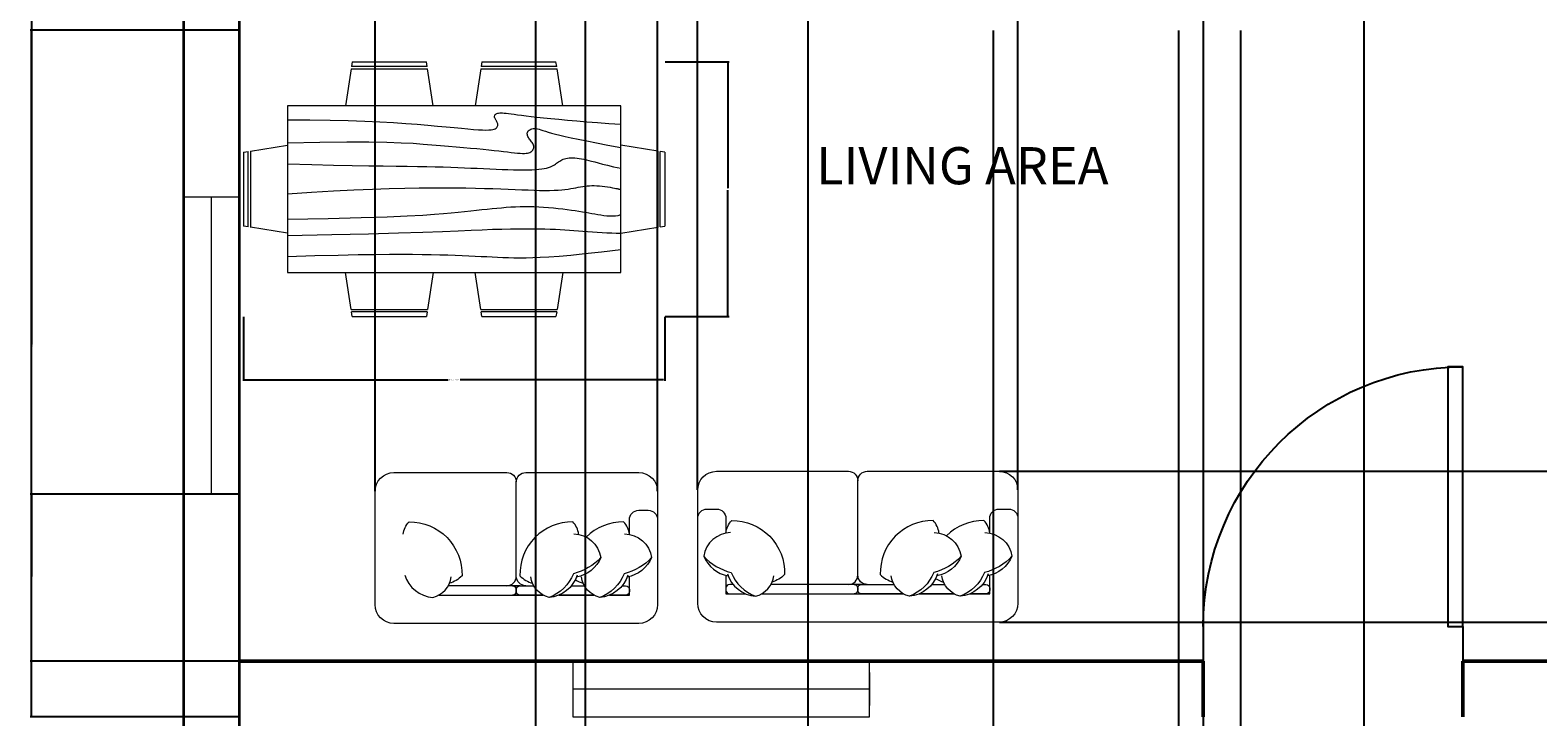
# Model space of a CAD drawing. Units: inches. Extents: x 8049 to 8459, y 820 to 1350.
# Tile 22 of 25: x 8050 to 8294, y 1046 to 1157. Entities that reach past the tile are written whole.
import ezdxf

# ---------------------------------------------------------------- set-up
doc = ezdxf.new("R2010")
doc.units = ezdxf.units.IN
doc.header["$MEASUREMENT"] = 0
for name, color, linetype, lineweight in [('A-ANNO-DIMS', 2, 'Continuous', 18), ('A-AREA-IDEN', 7, 'Continuous', 25), ('A-DOOR', 3, 'Continuous', 25), ('A-FURN', 8, 'Continuous', 18), ('A-GLAZ', 4, 'Continuous', 18), ('A-WALL', 7, 'Continuous', 50), ('C-SITE-WALL', 7, 'Continuous', 35)]:
    doc.layers.add(name, color=color, linetype=linetype, lineweight=lineweight)
doc.styles.get("Standard").update_dxf_attribs({"font": 'arial.ttf'})
doc.dimstyles.get("Standard").update_dxf_attribs({"dimtxt": 0.18, "dimasz": 0.18, "dimexe": 0.18, "dimexo": 0.0625, "dimgap": 0.09, "dimtad": 0, "dimtih": 1, "dimtoh": 1, "dimdec": 4, "dimzin": 0, "dimdsep": 46, "dimtxsty": 'Standard', "dimcen": 0.09, "dimadec": 0, "dimazin": 0, "dimtfac": 1, "dimtdec": 4, "dimtofl": 0, "dimtmove": 0, "dimatfit": 3, "dimfxl": 1, "dimtolj": 1, "dimtzin": 0, "dimarcsym": 0})

# ---------------------------------------------------------------- blocks, each defined once
blk = doc.blocks.new('*U2')
for p, q in [((0, 0), (0, -100)), ((750, 0), (750, -100))]:
    blk.add_line(p, q)
blk.add_lwpolyline([(0, 0), (0, 750), (43.75, 750), (43.75, 0)], close=True)
blk.add_arc((0, 0), 750, 0, 90)
blk = doc.blocks.new('*U4')
for p, q in [((0, 100), (0, 0)), ((900, 100), (900, 0)), ((0, 50), (900, 50))]:
    blk.add_line(p, q)
blk = doc.blocks.new('Dining Set - 36 x 72 in.')
for p, q in [((-22, 27.5), (-22.1562, 26.50042)), ((-5.8416, 26.5), (-22.1534, 26.5)), ((-22, 27.5), (-6, 27.5)), ((-5.8437, 26.49966), (-6, 27.5)), ((6, 27.5), (5.8438, 26.50042)), ((22.1584, 26.5), (5.8466, 26.5)), ((6, 27.5), (22, 27.5)), ((22.1563, 26.49966), (22, 27.5)), ((-22.2343, 26.00059), (-23.4847, 17.99762)), ((-22.2304, 26), (-5.7608, 26)), ((-4.5152, 17.99762), (-5.7655, 25.99926)), ((5.7657, 26.00059), (4.5153, 17.99762)), ((5.7696, 26), (22.2392, 26)), ((23.4848, 17.99762), (22.2345, 25.99926)), ((36, 18), (-36, 18)), ((-36, 18), (-36, -18)), ((36, -18), (36, 18)), ((-45.5, 8), (-44.5004, 8.15617)), ((-45.5, 8), (-45.5, -8)), ((-44.5, -8.15843), (-44.5, 8.15338)), ((-44.0006, 8.23428), (-35.9976, 9.48474)), ((-44, 8.23041), (-44, -8.23915)), ((44.0006, 8.23428), (35.9976, 9.48474)), ((44, 8.23041), (44, -8.23915)), ((44.5, -8.15843), (44.5, 8.15338)), ((45.5, 8), (44.5005, 8.15617)), ((45.5, 8), (45.5, -8)), ((-44.4997, -8.15631), (-45.5, -8)), ((-35.9976, -9.48476), (-43.9993, -8.2345)), ((35.9976, -9.48476), (43.9993, -8.2345)), ((44.4997, -8.15631), (45.5, -8)), ((-36, -18), (36, -18)), ((-22.2343, -26.0006), (-23.4847, -17.99762)), ((-4.5152, -17.99762), (-5.7655, -25.99928)), ((5.7657, -26.0006), (4.5153, -17.99762)), ((23.4848, -17.99762), (22.2345, -25.99928)), ((-22.2304, -26), (-5.7608, -26)), ((5.7696, -26), (22.2392, -26)), ((-22, -27.5), (-22.1562, -26.50044)), ((-5.8416, -26.5), (-22.1534, -26.5)), ((-22, -27.5), (-6, -27.5)), ((-5.8437, -26.49967), (-6, -27.5)), ((6, -27.5), (5.8438, -26.50044)), ((22.1584, -26.5), (5.8466, -26.5)), ((6, -27.5), (22, -27.5)), ((22.1563, -26.49967), (22, -27.5))]:
    blk.add_line(p, q)
for points in [[(-36, 15), (-31.1772, 14.97754), (-26.8079, 14.91406), (-22.8538, 14.81543), (-19.276, 14.6875), (-16.0362, 14.53613), (-13.0957, 14.36718), (-10.4159, 14.18652), (-7.9583, 14), (-5.6904, 13.81315), (-3.6035, 13.63021), (-1.6954, 13.45508), (0.0365, 13.29166), (1.5945, 13.14388), (2.9811, 13.01562), (4.1988, 12.9108), (5.25, 12.83333), (6.1393, 12.78613), (6.8802, 12.76823), (7.4883, 12.77767), (7.9792, 12.8125), (8.3685, 12.87077), (8.6719, 12.95052), (8.9049, 13.0498), (9.0833, 13.16666), (9.2205, 13.29899), (9.3216, 13.44401), (9.3895, 13.59879), (9.4271, 13.76041), (9.4373, 13.92594), (9.4232, 14.09245), (9.3875, 14.257), (9.3333, 14.41666), (9.2638, 14.56917), (9.1836, 14.71484), (9.0975, 14.85465), (9.0104, 14.98958), (8.9272, 15.1206), (8.8529, 15.2487), (8.7922, 15.37483), (8.75, 15.5), (8.7305, 15.62467), (8.7344, 15.74739), (8.7617, 15.86621), (8.8125, 15.97916), (8.8867, 16.08431), (8.9844, 16.17968), (9.1055, 16.26334), (9.25, 16.33333), (9.4189, 16.38802), (9.6172, 16.42708), (9.8506, 16.45052), (10.125, 16.45833), (10.4463, 16.45052), (10.8203, 16.42708), (11.2529, 16.38802), (11.75, 16.33333), (12.3184, 16.26318), (12.9694, 16.17838), (13.7151, 16.07991), (14.5677, 15.96875), (15.5395, 15.84586), (16.6426, 15.71224), (17.8893, 15.56884), (19.2917, 15.41666), (20.859, 15.25667), (22.5879, 15.08984), (24.4721, 14.91715), (26.5052, 14.73958), (28.6809, 14.5581), (30.9929, 14.3737), (33.4347, 14.18733), (36, 14)], [(-36, 10), (-28.9766, 10.14274), (-23.1725, 10.20442), (-18.4241, 10.19775), (-14.5677, 10.13541), (-11.4399, 10.03011), (-8.877, 9.89453), (-6.7154, 9.74137), (-4.7917, 9.58333), (-2.9698, 9.43082), (-1.2246, 9.28515), (0.4415, 9.14534), (2.026, 9.01041), (3.5266, 8.87939), (4.9408, 8.7513), (6.266, 8.62516), (7.5, 8.5), (8.6411, 8.37549), (9.6914, 8.2539), (10.6538, 8.13818), (11.5312, 8.03125), (12.3267, 7.93603), (13.043, 7.85547), (13.6831, 7.79248), (14.25, 7.75), (14.7471, 7.7303), (15.1797, 7.73307), (15.5537, 7.75732), (15.875, 7.80208), (16.1494, 7.86637), (16.3828, 7.94922), (16.5811, 8.04964), (16.75, 8.16666), (16.8944, 8.29915), (17.0143, 8.44531), (17.1089, 8.60319), (17.1771, 8.77083), (17.218, 8.94629), (17.2305, 9.1276), (17.2137, 9.31282), (17.1667, 9.5), (17.0895, 9.6875), (16.987, 9.875), (16.8649, 10.0625), (16.7292, 10.25), (16.5856, 10.4375), (16.4401, 10.625), (16.2985, 10.8125), (16.1667, 11), (16.05, 11.18733), (15.9518, 11.3737), (15.8752, 11.5581), (15.8229, 11.73958), (15.798, 11.91715), (15.8034, 12.08984), (15.842, 12.25667), (15.9167, 12.41666), (16.0295, 12.56836), (16.1784, 12.70833), (16.3605, 12.83268), (16.5729, 12.9375), (16.8127, 13.01888), (17.0768, 13.07291), (17.3625, 13.0957), (17.6667, 13.08333), (17.9894, 13.03312), (18.3418, 12.94726), (18.7382, 12.82918), (19.1927, 12.68229), (19.7195, 12.51001), (20.3327, 12.31575), (21.0465, 12.10294), (21.875, 11.875), (22.8357, 11.63354), (23.959, 11.37304), (25.2786, 11.08618), (26.8282, 10.76562), (28.6414, 10.40405), (30.752, 9.99414), (33.1936, 9.52856), (36, 9)], [(-36, 5.5), (-30.7157, 5.3348), (-26.069, 5.20963), (-21.9946, 5.11767), (-18.4271, 5.05208), (-15.3009, 5.00602), (-12.5508, 4.97265), (-10.1112, 4.94515), (-7.9167, 4.91666), (-5.909, 4.88167), (-4.0586, 4.83984), (-2.3429, 4.79215), (-0.7396, 4.73958), (0.7739, 4.6831), (2.22, 4.6237), (3.6213, 4.56233), (5, 4.5), (6.373, 4.43782), (7.7344, 4.3776), (9.0723, 4.32129), (10.375, 4.27083), (11.6309, 4.22819), (12.8281, 4.19531), (13.9551, 4.17415), (15, 4.16666), (15.954, 4.17448), (16.819, 4.19791), (17.6001, 4.23698), (18.3021, 4.29166), (18.9299, 4.36198), (19.4883, 4.44791), (19.9823, 4.54948), (20.4167, 4.66666), (20.7969, 4.79899), (21.1302, 4.94401), (21.4245, 5.09879), (21.6875, 5.26041), (21.9271, 5.42594), (22.1511, 5.59245), (22.3672, 5.757), (22.5834, 5.91666), (22.8065, 6.06868), (23.0404, 6.21093), (23.2879, 6.34147), (23.5521, 6.45833), (23.8358, 6.55957), (24.142, 6.64323), (24.4735, 6.70735), (24.8334, 6.75), (25.2235, 6.76969), (25.642, 6.76692), (26.0858, 6.74267), (26.5521, 6.69791), (27.0379, 6.63362), (27.5404, 6.55078), (28.0565, 6.45036), (28.5834, 6.33333), (29.1242, 6.19987), (29.7071, 6.04687), (30.3661, 5.87044), (31.1354, 5.66666), (32.0493, 5.43164), (33.142, 5.16146), (34.4475, 4.85221), (36, 4.5)], [(-36, -1), (-30.7915, -0.6591), (-26.0195, -0.38216), (-21.6519, -0.16284), (-17.6563, 0.00521), (-14.0005, 0.12833), (-10.6523, 0.21289), (-7.5796, 0.26522), (-4.75, 0.29166), (-2.134, 0.29793), (0.2878, 0.28711), (2.5317, 0.26163), (4.6146, 0.22396), (6.5529, 0.17651), (8.3633, 0.12174), (10.0623, 0.06209), (11.6667, 0), (13.1899, -0.06201), (14.6341, -0.1211), (15.9982, -0.17432), (17.2813, -0.21875), (18.4823, -0.25147), (19.6003, -0.26953), (20.6343, -0.27002), (21.5834, -0.25), (22.4481, -0.20768), (23.2357, -0.14584), (23.9549, -0.06836), (24.6146, 0.02083), (25.2235, 0.11784), (25.7904, 0.21875), (26.3241, 0.31966), (26.8334, 0.41666), (27.3265, 0.50618), (27.8099, 0.58593), (28.2894, 0.65397), (28.7709, 0.70833), (29.2601, 0.74707), (29.763, 0.76823), (30.2855, 0.76985), (30.8334, 0.75), (31.4088, 0.70784), (31.9994, 0.64713), (32.589, 0.57275), (33.1615, 0.48958), (33.7008, 0.4025), (34.1908, 0.3164), (34.6153, 0.23616), (34.9584, 0.16666), (35.2099, 0.11165), (35.3848, 0.07031), (35.504, 0.04069), (35.5886, 0.02083), (35.6594, 0.00879), (35.7377, 0.0026), (35.8442, 0.00032), (36, 0)], [(-36, -6.5), (-27.1843, -6.31267), (-20.084, -6.1263), (-14.469, -5.9419), (-10.1094, -5.76042), (-6.7752, -5.58285), (-4.2363, -5.41016), (-2.2629, -5.24333), (-0.625, -5.08334), (0.8708, -4.93099), (2.2715, -4.78646), (3.5872, -4.64974), (4.8281, -4.52084), (6.0046, -4.39974), (7.127, -4.28646), (8.2053, -4.18099), (9.25, -4.08334), (10.2705, -3.99382), (11.2734, -3.91407), (12.2647, -3.84603), (13.25, -3.79167), (14.2354, -3.75293), (15.2266, -3.73177), (16.2295, -3.73015), (17.25, -3.75), (18.2912, -3.79248), (19.3451, -3.85547), (20.4009, -3.93604), (21.4479, -4.03125), (22.4754, -4.13819), (23.4727, -4.25391), (24.4289, -4.37549), (25.3334, -4.5), (26.1785, -4.62492), (26.9694, -4.74935), (27.7145, -4.87281), (28.4219, -4.99479), (29.1, -5.11483), (29.7572, -5.23242), (30.4016, -5.34709), (31.0417, -5.45834), (31.6837, -5.56437), (32.3262, -5.65821), (32.9658, -5.73153), (33.599, -5.77604), (34.2224, -5.78345), (34.8327, -5.74545), (35.4264, -5.65373), (36, -5.5)], [(-36, -10), (-26.4022, -9.81299), (-18.4675, -9.62891), (-11.9839, -9.45069), (-6.7396, -9.28125), (-2.5226, -9.12354), (0.8789, -8.98047), (3.6769, -8.85498), (6.0833, -8.75), (8.2767, -8.66765), (10.3021, -8.60677), (12.1712, -8.56543), (13.8958, -8.54167), (15.4876, -8.53353), (16.9583, -8.53907), (18.3197, -8.55632), (19.5834, -8.58334), (20.7616, -8.61841), (21.8685, -8.66081), (22.9188, -8.71004), (23.9271, -8.76563), (24.9081, -8.82707), (25.8763, -8.89388), (26.8465, -8.96558), (27.8334, -9.04167), (28.8474, -9.12118), (29.8828, -9.20117), (30.93, -9.27824), (31.9792, -9.34896), (33.0205, -9.40991), (34.0443, -9.45768), (35.0407, -9.48885), (36, -9.5)], [(-36, -14.5), (-30.0881, -14.33513), (-25.0332, -14.21224), (-20.7312, -14.12647), (-17.0781, -14.07292), (-13.97, -14.04671), (-11.3027, -14.04297), (-8.9724, -14.05681), (-6.875, -14.08334), (-4.9224, -14.11833), (-3.0905, -14.16016), (-1.3709, -14.20785), (0.2448, -14.26042), (1.7647, -14.3169), (3.1973, -14.3763), (4.5507, -14.43767), (5.8333, -14.5), (7.0554, -14.5621), (8.235, -14.62175), (9.3922, -14.67652), (10.5469, -14.72396), (11.7192, -14.76164), (12.929, -14.78711), (14.1965, -14.79794), (15.5417, -14.79167), (16.9933, -14.76424), (18.6152, -14.70508), (20.4804, -14.60197), (22.6615, -14.44271), (25.2312, -14.21509), (28.2624, -13.9069), (31.8277, -13.50594), (36, -13)]]:
    blk.add_lwpolyline(points)
blk = doc.blocks.new('WIN-48IN-SURROUND')
for p, q in [((9, 48), (0, 48)), ((0, 48), (0, 0)), ((0, 0), (9, 0))]:
    blk.add_line(p, q)
blk = doc.blocks.new('*D42')
at = {"layer": 'A-ANNO-DIMS', "color": 0, "lineweight": -2, "transparency": 16777216}
for p, q in [((8084.11, 1110.51), (8084.11, 1100.17)), ((8152.26, 1110.51), (8152.26, 1100.17)), ((8084.29, 1100.35), (8117.22, 1100.35)), ((8152.08, 1100.35), (8119.16, 1100.35))]:
    blk.add_line(p, q, dxfattribs=at)
at = {"layer": 'A-ANNO-DIMS', "color": 0, "transparency": 16777216}
for points in [[(8084.29, 1100.38), (8084.29, 1100.32), (8084.11, 1100.35)], [(8152.08, 1100.38), (8152.08, 1100.32), (8152.26, 1100.35)]]:
    blk.add_solid(points, dxfattribs=at)
at = {"layer": 'Defpoints', "color": 0, "transparency": 16777216}
for p in [(8084.11, 1110.57), (8152.26, 1110.57), (8152.26, 1100.35)]:
    blk.add_point(p, dxfattribs=at)
at = {"layer": 'A-ANNO-DIMS', "color": 0, "transparency": 16777216, "insert": (8118.19, 1100.35), "char_height": 0.18, "attachment_point": 5}
blk.add_mtext('\\A1;DINING SET 68', dxfattribs=at)
blk = doc.blocks.new('*D43')
at = {"layer": 'A-ANNO-DIMS', "color": 0, "lineweight": -2, "transparency": 16777216}
for p, q in [((8152.33, 1151.76), (8162.67, 1151.76)), ((8162.49, 1151.58), (8162.49, 1131.35)), ((8162.49, 1110.75), (8162.49, 1130.99)), ((8152.33, 1110.57), (8162.67, 1110.57))]:
    blk.add_line(p, q, dxfattribs=at)
at = {"layer": 'A-ANNO-DIMS', "color": 0, "transparency": 16777216}
for points in [[(8162.46, 1151.58), (8162.52, 1151.58), (8162.49, 1151.76)], [(8162.46, 1110.75), (8162.52, 1110.75), (8162.49, 1110.57)]]:
    blk.add_solid(points, dxfattribs=at)
at = {"layer": 'Defpoints', "color": 0, "transparency": 16777216}
for p in [(8152.26, 1151.76), (8162.49, 1151.76), (8152.26, 1110.57)]:
    blk.add_point(p, dxfattribs=at)
at = {"layer": 'A-ANNO-DIMS', "color": 0, "transparency": 16777216, "insert": (8162.49, 1131.17), "char_height": 0.18, "attachment_point": 5}
blk.add_mtext('\\A1;41', dxfattribs=at)
blk = doc.blocks.new('*D51')
at = {"layer": 'A-ANNO-DIMS', "color": 0, "lineweight": -2, "transparency": 16777216}
for p, q in [((8083.33, 1267.87), (8049.62, 1267.87)), ((8049.8, 1267.69), (8049.8, 1157.05)), ((8049.8, 1046.05), (8049.8, 1156.69)), ((8083.33, 1045.87), (8049.62, 1045.87))]:
    blk.add_line(p, q, dxfattribs=at)
at = {"layer": 'A-ANNO-DIMS', "color": 0, "transparency": 16777216}
for points in [[(8049.77, 1267.69), (8049.83, 1267.69), (8049.8, 1267.87)], [(8049.77, 1046.05), (8049.83, 1046.05), (8049.8, 1045.87)]]:
    blk.add_solid(points, dxfattribs=at)
at = {"layer": 'Defpoints', "color": 0, "transparency": 16777216}
for p in [(8049.8, 1267.87), (8083.4, 1267.87), (8083.4, 1045.87)]:
    blk.add_point(p, dxfattribs=at)
at = {"layer": 'A-ANNO-DIMS', "color": 0, "transparency": 16777216, "insert": (8049.8, 1156.87), "char_height": 0.18, "attachment_point": 5}
blk.add_mtext('\\A1;222', dxfattribs=at)
blk = doc.blocks.new('*D56')
at = {"layer": 'A-ANNO-DIMS', "color": 0, "lineweight": -2, "transparency": 16777216}
for p, q in [((8205.4, 1156.81), (8205.4, 820.09)), ((8235.4, 1156.81), (8235.4, 820.09)), ((8205.58, 820.27), (8220.18, 820.27)), ((8235.22, 820.27), (8220.62, 820.27))]:
    blk.add_line(p, q, dxfattribs=at)
at = {"layer": 'A-ANNO-DIMS', "color": 0, "transparency": 16777216}
for points in [[(8205.58, 820.3), (8205.58, 820.24), (8205.4, 820.27)], [(8235.22, 820.3), (8235.22, 820.24), (8235.4, 820.27)]]:
    blk.add_solid(points, dxfattribs=at)
at = {"layer": 'Defpoints', "color": 0, "transparency": 16777216}
for p in [(8205.4, 1156.87), (8235.4, 1156.87), (8235.4, 820.27)]:
    blk.add_point(p, dxfattribs=at)
at = {"layer": 'A-ANNO-DIMS', "color": 0, "transparency": 16777216, "insert": (8220.4, 820.27), "char_height": 0.18, "attachment_point": 5}
blk.add_mtext('\\A1;30', dxfattribs=at)
blk = doc.blocks.new('*D58')
at = {"layer": 'A-ANNO-DIMS', "color": 0, "lineweight": -2, "transparency": 16777216}
for p, q in [((8139.4, 1162.81), (8139.4, 820.09)), ((8175.4, 1162.81), (8175.4, 820.09)), ((8139.58, 820.27), (8157.18, 820.27)), ((8175.22, 820.27), (8157.62, 820.27))]:
    blk.add_line(p, q, dxfattribs=at)
at = {"layer": 'A-ANNO-DIMS', "color": 0, "transparency": 16777216}
for points in [[(8139.58, 820.3), (8139.58, 820.24), (8139.4, 820.27)], [(8175.22, 820.3), (8175.22, 820.24), (8175.4, 820.27)]]:
    blk.add_solid(points, dxfattribs=at)
at = {"layer": 'Defpoints', "color": 0, "transparency": 16777216}
for p in [(8139.4, 1162.87), (8175.4, 1162.87), (8175.4, 820.27)]:
    blk.add_point(p, dxfattribs=at)
at = {"layer": 'A-ANNO-DIMS', "color": 0, "transparency": 16777216, "insert": (8157.4, 820.27), "char_height": 0.18, "attachment_point": 5}
blk.add_mtext('\\A1;36', dxfattribs=at)
blk = doc.blocks.new('*D59')
at = {"layer": 'A-ANNO-DIMS', "color": 0, "lineweight": -2, "transparency": 16777216}
for p, q in [((8083.4, 925.93), (8083.4, 1349.65)), ((8083.58, 1349.47), (8107.17, 1349.47)), ((8131.22, 1349.47), (8107.62, 1349.47)), ((8131.4, 925.93), (8131.4, 1349.65))]:
    blk.add_line(p, q, dxfattribs=at)
at = {"layer": 'A-ANNO-DIMS', "color": 0, "transparency": 16777216}
for points in [[(8083.58, 1349.5), (8083.58, 1349.44), (8083.4, 1349.47)], [(8131.22, 1349.5), (8131.22, 1349.44), (8131.4, 1349.47)]]:
    blk.add_solid(points, dxfattribs=at)
at = {"layer": 'Defpoints', "color": 0, "transparency": 16777216}
for p in [(8131.4, 1349.47), (8083.4, 925.87), (8131.4, 925.87)]:
    blk.add_point(p, dxfattribs=at)
at = {"layer": 'A-ANNO-DIMS', "color": 0, "transparency": 16777216, "insert": (8107.4, 1349.47), "char_height": 0.18, "attachment_point": 5}
blk.add_mtext('\\A1;48', dxfattribs=at)
blk = doc.blocks.new('*D72')
at = {"layer": 'A-ANNO-DIMS', "color": 0, "lineweight": -2, "transparency": 16777216}
for p, q in [((8083.33, 1081.87), (8049.62, 1081.87)), ((8049.8, 1081.69), (8049.8, 1068.55)), ((8049.8, 1055.05), (8049.8, 1068.19)), ((8083.33, 1054.87), (8049.62, 1054.87))]:
    blk.add_line(p, q, dxfattribs=at)
at = {"layer": 'A-ANNO-DIMS', "color": 0, "transparency": 16777216}
for points in [[(8049.77, 1081.69), (8049.83, 1081.69), (8049.8, 1081.87)], [(8049.77, 1055.05), (8049.83, 1055.05), (8049.8, 1054.87)]]:
    blk.add_solid(points, dxfattribs=at)
at = {"layer": 'Defpoints', "color": 0, "transparency": 16777216}
for p in [(8049.8, 1081.87), (8083.4, 1081.87), (8083.4, 1054.87)]:
    blk.add_point(p, dxfattribs=at)
at = {"layer": 'A-ANNO-DIMS', "color": 0, "transparency": 16777216, "insert": (8049.8, 1068.37), "char_height": 0.18, "attachment_point": 5}
blk.add_mtext('\\A1;27', dxfattribs=at)
blk = doc.blocks.new('*D73')
at = {"layer": 'A-ANNO-DIMS', "color": 0, "lineweight": -2, "transparency": 16777216}
for p, q in [((8239.4, 1204.81), (8239.4, 820.09)), ((8265.4, 1204.81), (8265.4, 820.09)), ((8239.58, 820.27), (8252.18, 820.27)), ((8265.22, 820.27), (8252.62, 820.27))]:
    blk.add_line(p, q, dxfattribs=at)
at = {"layer": 'A-ANNO-DIMS', "color": 0, "transparency": 16777216}
for points in [[(8239.58, 820.3), (8239.58, 820.24), (8239.4, 820.27)], [(8265.22, 820.3), (8265.22, 820.24), (8265.4, 820.27)]]:
    blk.add_solid(points, dxfattribs=at)
at = {"layer": 'Defpoints', "color": 0, "transparency": 16777216}
for p in [(8239.4, 1204.87), (8265.4, 1204.87), (8265.4, 820.27)]:
    blk.add_point(p, dxfattribs=at)
at = {"layer": 'A-ANNO-DIMS', "color": 0, "transparency": 16777216, "insert": (8252.4, 820.27), "char_height": 0.18, "attachment_point": 5}
blk.add_mtext('\\A1;26', dxfattribs=at)
blk = doc.blocks.new('*D75')
at = {"layer": 'A-ANNO-DIMS', "color": 0, "lineweight": -2, "transparency": 16777216}
for p, q in [((8239.4, 1162.81), (8239.4, 820.09)), ((8245.4, 1156.81), (8245.4, 820.09)), ((8239.58, 820.27), (8242.25, 820.27)), ((8245.22, 820.27), (8242.55, 820.27))]:
    blk.add_line(p, q, dxfattribs=at)
at = {"layer": 'A-ANNO-DIMS', "color": 0, "transparency": 16777216}
for points in [[(8239.58, 820.3), (8239.58, 820.24), (8239.4, 820.27)], [(8245.22, 820.3), (8245.22, 820.24), (8245.4, 820.27)]]:
    blk.add_solid(points, dxfattribs=at)
at = {"layer": 'Defpoints', "color": 0, "transparency": 16777216}
for p in [(8239.4, 1162.87), (8245.4, 1156.87), (8245.4, 820.27)]:
    blk.add_point(p, dxfattribs=at)
at = {"layer": 'A-ANNO-DIMS', "color": 0, "transparency": 16777216, "insert": (8242.4, 820.27), "char_height": 0.18, "attachment_point": 5}
blk.add_mtext('\\A1;6', dxfattribs=at)
blk = doc.blocks.new('*D76')
at = {"layer": 'A-ANNO-DIMS', "color": 0, "lineweight": -2, "transparency": 16777216}
for p, q in [((8083.4, 1054.81), (8083.4, 820.09)), ((8299.4, 1054.81), (8299.4, 820.09)), ((8083.58, 820.27), (8191.11, 820.27)), ((8299.22, 820.27), (8191.69, 820.27))]:
    blk.add_line(p, q, dxfattribs=at)
at = {"layer": 'A-ANNO-DIMS', "color": 0, "transparency": 16777216}
for points in [[(8083.58, 820.3), (8083.58, 820.24), (8083.4, 820.27)], [(8299.22, 820.3), (8299.22, 820.24), (8299.4, 820.27)]]:
    blk.add_solid(points, dxfattribs=at)
at = {"layer": 'Defpoints', "color": 0, "transparency": 16777216}
for p in [(8083.4, 1054.87), (8299.4, 1054.87), (8299.4, 820.27)]:
    blk.add_point(p, dxfattribs=at)
at = {"layer": 'A-ANNO-DIMS', "color": 0, "transparency": 16777216, "insert": (8191.4, 820.27), "char_height": 0.18, "attachment_point": 5}
blk.add_mtext('\\A1;216', dxfattribs=at)
blk = doc.blocks.new('*D77')
at = {"layer": 'A-ANNO-DIMS', "color": 0, "lineweight": -2, "transparency": 16777216}
for p, q in [((8083.33, 1156.87), (8049.62, 1156.87)), ((8049.8, 1156.69), (8049.8, 1106.05)), ((8049.8, 1055.05), (8049.8, 1105.69)), ((8083.33, 1054.87), (8049.62, 1054.87))]:
    blk.add_line(p, q, dxfattribs=at)
at = {"layer": 'A-ANNO-DIMS', "color": 0, "transparency": 16777216}
for points in [[(8049.77, 1156.69), (8049.83, 1156.69), (8049.8, 1156.87)], [(8049.77, 1055.05), (8049.83, 1055.05), (8049.8, 1054.87)]]:
    blk.add_solid(points, dxfattribs=at)
at = {"layer": 'Defpoints', "color": 0, "transparency": 16777216}
for p in [(8049.8, 1156.87), (8083.4, 1156.87), (8083.4, 1054.87)]:
    blk.add_point(p, dxfattribs=at)
at = {"layer": 'A-ANNO-DIMS', "color": 0, "transparency": 16777216, "insert": (8049.8, 1105.87), "char_height": 0.18, "attachment_point": 5}
blk.add_mtext('\\A1;102', dxfattribs=at)
blk = doc.blocks.new('*D78')
at = {"layer": 'A-ANNO-DIMS', "color": 0, "lineweight": -2, "transparency": 16777216}
for p, q in [((8105.39, 1082.37), (8105.39, 1349.65)), ((8105.57, 1349.47), (8127.86, 1349.47)), ((8150.94, 1349.47), (8128.65, 1349.47)), ((8151.12, 1082.37), (8151.12, 1349.65))]:
    blk.add_line(p, q, dxfattribs=at)
at = {"layer": 'A-ANNO-DIMS', "color": 0, "transparency": 16777216}
for points in [[(8105.57, 1349.5), (8105.57, 1349.44), (8105.39, 1349.47)], [(8150.94, 1349.5), (8150.94, 1349.44), (8151.12, 1349.47)]]:
    blk.add_solid(points, dxfattribs=at)
at = {"layer": 'Defpoints', "color": 0, "transparency": 16777216}
for p in [(8151.12, 1349.47), (8105.39, 1082.31), (8151.12, 1082.31)]:
    blk.add_point(p, dxfattribs=at)
at = {"layer": 'A-ANNO-DIMS', "color": 0, "transparency": 16777216, "insert": (8128.25, 1349.47), "char_height": 0.18, "attachment_point": 5}
blk.add_mtext('\\A1;45.72', dxfattribs=at)
blk = doc.blocks.new('*D79')
at = {"layer": 'A-ANNO-DIMS', "color": 0, "lineweight": -2, "transparency": 16777216}
for p, q in [((8157.59, 1082.57), (8157.59, 1349.65)), ((8157.77, 1349.47), (8183.11, 1349.47)), ((8209.23, 1349.47), (8183.9, 1349.47)), ((8209.41, 1082.57), (8209.41, 1349.65))]:
    blk.add_line(p, q, dxfattribs=at)
at = {"layer": 'A-ANNO-DIMS', "color": 0, "transparency": 16777216}
for points in [[(8157.77, 1349.5), (8157.77, 1349.44), (8157.59, 1349.47)], [(8209.23, 1349.5), (8209.23, 1349.44), (8209.41, 1349.47)]]:
    blk.add_solid(points, dxfattribs=at)
at = {"layer": 'Defpoints', "color": 0, "transparency": 16777216}
for p in [(8209.41, 1349.47), (8157.59, 1082.51), (8209.41, 1082.51)]:
    blk.add_point(p, dxfattribs=at)
at = {"layer": 'A-ANNO-DIMS', "color": 0, "transparency": 16777216, "insert": (8183.5, 1349.47), "char_height": 0.18, "attachment_point": 5}
blk.add_mtext('\\A1;51.82', dxfattribs=at)
blk = doc.blocks.new('*D80')
at = {"layer": 'A-ANNO-DIMS', "color": 0, "lineweight": -2, "transparency": 16777216}
for p, q in [((8206.43, 1085.56), (8459.18, 1085.56)), ((8459, 1085.38), (8459, 1073.55)), ((8459, 1061.35), (8459, 1073.19)), ((8206.43, 1061.17), (8459.18, 1061.17))]:
    blk.add_line(p, q, dxfattribs=at)
at = {"layer": 'A-ANNO-DIMS', "color": 0, "transparency": 16777216}
for points in [[(8458.97, 1085.38), (8459.03, 1085.38), (8459, 1085.56)], [(8458.97, 1061.35), (8459.03, 1061.35), (8459, 1061.17)]]:
    blk.add_solid(points, dxfattribs=at)
at = {"layer": 'Defpoints', "color": 0, "transparency": 16777216}
for p in [(8206.37, 1085.56), (8459, 1085.56), (8206.37, 1061.17)]:
    blk.add_point(p, dxfattribs=at)
at = {"layer": 'A-ANNO-DIMS', "color": 0, "transparency": 16777216, "insert": (8459, 1073.37), "char_height": 0.18, "attachment_point": 5}
blk.add_mtext('\\A1;24.386', dxfattribs=at)
blk = doc.blocks.new('*D86')
at = {"layer": 'A-ANNO-DIMS', "color": 0, "lineweight": -2, "transparency": 16777216}
for p, q in [((8265.4, 1204.81), (8265.4, 820.09)), ((8295.4, 1204.81), (8295.4, 820.09)), ((8265.58, 820.27), (8280.18, 820.27)), ((8295.22, 820.27), (8280.62, 820.27))]:
    blk.add_line(p, q, dxfattribs=at)
at = {"layer": 'A-ANNO-DIMS', "color": 0, "transparency": 16777216}
for points in [[(8265.58, 820.3), (8265.58, 820.24), (8265.4, 820.27)], [(8295.22, 820.3), (8295.22, 820.24), (8295.4, 820.27)]]:
    blk.add_solid(points, dxfattribs=at)
at = {"layer": 'Defpoints', "color": 0, "transparency": 16777216}
for p in [(8265.4, 1204.87), (8295.4, 1204.87), (8295.4, 820.27)]:
    blk.add_point(p, dxfattribs=at)
at = {"layer": 'A-ANNO-DIMS', "color": 0, "transparency": 16777216, "insert": (8280.4, 820.27), "char_height": 0.18, "attachment_point": 5}
blk.add_mtext('\\A1;30', dxfattribs=at)
blk = doc.blocks.new('*D88')
at = {"layer": 'A-ANNO-DIMS', "color": 0, "lineweight": -2, "transparency": 16777216}
for p, q in [((8083.4, 1162.81), (8083.4, 820.09)), ((8139.4, 1162.81), (8139.4, 820.09)), ((8083.58, 820.27), (8111.18, 820.27)), ((8139.22, 820.27), (8111.62, 820.27))]:
    blk.add_line(p, q, dxfattribs=at)
at = {"layer": 'A-ANNO-DIMS', "color": 0, "transparency": 16777216}
for points in [[(8083.58, 820.3), (8083.58, 820.24), (8083.4, 820.27)], [(8139.22, 820.3), (8139.22, 820.24), (8139.4, 820.27)]]:
    blk.add_solid(points, dxfattribs=at)
at = {"layer": 'Defpoints', "color": 0, "transparency": 16777216}
for p in [(8083.4, 1162.87), (8139.4, 1162.87), (8139.4, 820.27)]:
    blk.add_point(p, dxfattribs=at)
at = {"layer": 'A-ANNO-DIMS', "color": 0, "transparency": 16777216, "insert": (8111.4, 820.27), "char_height": 0.18, "attachment_point": 5}
blk.add_mtext('\\A1;56', dxfattribs=at)

msp = doc.modelspace()

# ---------------------------------------------------------------- linework, layer by layer
at = {"layer": 'A-FURN', "ltscale": 0.03}
for points in [[(8181.98, 1085.5602, -0.41421356), (8183.5041, 1084.0361, -0.41421356), (8185.0283, 1085.5602), (8206.3663, 1085.5602, -0.41421356), (8209.4146, 1082.5119), (8209.4146, 1064.2222, -0.41421356), (8206.3663, 1061.1739), (8160.642, 1061.1739, -0.41421356), (8157.5937, 1064.2222), (8157.5937, 1082.5119, -0.41421356), (8160.642, 1085.5602), (8181.98, 1085.5602, -0.41421356), (8183.5041, 1084.0361, -0.41421356), (8185.0283, 1085.5602)], [(8126.7291, 1085.3555, -0.41421356), (8128.2532, 1083.8313, -0.41421356), (8129.7773, 1085.3555), (8148.0671, 1085.3555, -0.41421356), (8151.1153, 1082.3072), (8151.1153, 1064.0175, -0.41421356), (8148.0671, 1060.9692), (8108.4394, 1060.9692, -0.41421356), (8105.3911, 1064.0175), (8105.3911, 1082.3072, -0.41421356), (8108.4394, 1085.3555), (8126.7291, 1085.3555, -0.41421356), (8128.2532, 1083.8313, -0.41421356), (8129.7773, 1085.3555)]]:
    msp.add_lwpolyline(points, format="xyb", dxfattribs=at)
at = {"layer": 'A-FURN'}
for points in [[(8126.7291, 1067.0657, 0.41421356), (8128.2532, 1068.5899), (8128.2532, 1083.8313, 0.41421356)], [(8129.7773, 1067.0657, -0.41421356), (8128.2532, 1068.5899), (8128.2532, 1083.8313, -0.41421356)], [(8181.98, 1067.2705, 0.41421356), (8183.5041, 1068.7947), (8183.5041, 1084.0361, 0.41421356)], [(8185.0283, 1067.2705, -0.41421356), (8183.5041, 1068.7947), (8183.5041, 1084.0361, -0.41421356)], [(8146.5429, 1075.3733), (8146.5429, 1077.7347, -0.41421356), (8148.0671, 1079.2589), (8149.5912, 1079.2589, -0.41421356), (8151.1153, 1077.7347)], [(8157.5937, 1077.9395, -0.41421356), (8159.1179, 1079.4636), (8160.642, 1079.4636, -0.41421356), (8162.1662, 1077.9395), (8162.1662, 1075.5781)], [(8204.8421, 1075.5781), (8204.8421, 1077.9395, -0.41421356), (8206.3663, 1079.4636), (8207.8904, 1079.4636, -0.41421356), (8209.4146, 1077.9395)], [(8109.9602, 1075.3726, -0.16554063), (8110.9031, 1077.3864, -0.42598917), (8119.4629, 1068.6551, -0.12152332), (8117.431, 1067.4517, 7.11546429)], [(8138.3357, 1075.3726, 0.16554063), (8137.3929, 1077.3864, 0.42598917), (8128.833, 1068.6551, 0.12152332), (8130.8649, 1067.4517, -7.11546429)], [(8146.5462, 1075.3726, 0.16554063), (8145.6033, 1077.3864, 0.20023115), (8139.5531, 1074.9338, 0.12152332)], [(8162.1628, 1075.5774, -0.16554063), (8163.1057, 1077.5912, -0.42598917), (8171.6656, 1068.8599, -0.12152332), (8169.6336, 1067.6564, 7.11546429)], [(8196.635, 1075.5774, 0.16554063), (8195.6921, 1077.5912, 0.42598917), (8187.1322, 1068.8599, 0.12152332), (8189.1641, 1067.6564, -7.11546429)], [(8204.8455, 1075.5774, 0.16554063), (8203.9026, 1077.5912, 0.20023115), (8197.8523, 1075.1385, 0.12152332)], [(8137.5675, 1075.4655, -0.35677236), (8141.9348, 1071.6238, -0.24954205), (8137.9777, 1068.4578, 9.61688035)], [(8145.778, 1075.4655, -0.35677236), (8150.1453, 1071.6238, -0.24954205), (8146.1882, 1068.4578, 9.61688035)], [(8162.931, 1075.6703, 0.35677236), (8158.5637, 1071.8285, 0.24954205), (8162.5209, 1068.6626, -9.61688035)], [(8195.8668, 1075.6703, -0.35677236), (8200.2341, 1071.8285, -0.24954205), (8196.2769, 1068.6626, 9.61688035)], [(8204.0773, 1075.6703, -0.35677236), (8208.4445, 1071.8285, -0.24954205), (8204.4874, 1068.6626, 9.61688035)], [(8141.9348, 1071.6238, -0.14772988), (8137.4802, 1069.0044, -0.21334276), (8133.5496, 1065.1626, -0.17866181)], [(8150.1453, 1071.6238, -0.14772988), (8145.6907, 1069.0044, -0.21334276), (8141.7601, 1065.1626, -0.17866181)], [(8158.5637, 1071.8285, 0.14772988), (8163.0184, 1069.2091, 0.21334276), (8166.9489, 1065.3674, 0.17866181)], [(8200.2341, 1071.8285, -0.14772988), (8195.7794, 1069.2091, -0.21334276), (8191.8489, 1065.3674, -0.17866181)], [(8208.4445, 1071.8285, -0.14772988), (8203.9899, 1069.2091, -0.21334276), (8200.0594, 1065.3674, -0.17866181)], [(8110.2003, 1068.7956, 0.30666349), (8114.7463, 1065.1626, 0.30632997), (8117.716, 1068.4805, -0.87284716)], [(8126.7291, 1067.0657, 0.41421356), (8128.2532, 1068.5899)], [(8129.7773, 1067.0657, -0.41421356), (8128.2532, 1068.5899)], [(8138.0956, 1068.7956, -0.30666349), (8133.5496, 1065.1626, -0.30632997), (8130.5799, 1068.4805, 0.87284716)], [(8146.3061, 1068.7956, -0.30666349), (8141.7601, 1065.1626, -0.30632997), (8138.7904, 1068.4805, 0.87284716)], [(8143.3365, 1065.5416), (8146.5429, 1065.5416), (8146.5429, 1068.5369, -0.41421356)], [(8162.403, 1069.0004, 0.30666349), (8166.9489, 1065.3674, 0.30632997), (8169.9187, 1068.6852, -0.87284716)], [(8181.98, 1067.2705, 0.41421356), (8183.5041, 1068.7947)], [(8185.0283, 1067.2705, -0.41421356), (8183.5041, 1068.7947)], [(8196.3948, 1069.0004, -0.30666349), (8191.8489, 1065.3674, -0.30632997), (8188.8791, 1068.6852, 0.87284716)], [(8204.6053, 1069.0004, -0.30666349), (8200.0594, 1065.3674, -0.30632997), (8197.0896, 1068.6852, 0.87284716)], [(8201.6358, 1065.7464), (8204.8421, 1065.7464), (8204.8421, 1068.7417, -0.41421356)], [(8115.7055, 1065.5416), (8127.6435, 1065.5416, 0.41421356), (8128.2532, 1066.1513), (8128.2532, 1066.4561, 0.41421356), (8127.6435, 1067.0657), (8117.2402, 1067.0657, 0.41421356)], [(8132.5904, 1065.5416), (8128.8629, 1065.5416, -0.41421356), (8128.2532, 1066.1513), (8128.2532, 1066.4561, -0.41421356), (8128.8629, 1067.0657), (8131.0557, 1067.0657, -0.41421356)], [(8137.1693, 1067.0657), (8139.2662, 1067.0657, -0.41421356)], [(8137.7976, 1068.0475, 0.07186538), (8139.0754, 1067.4517, -7.11546429)], [(8145.3798, 1067.0657), (8145.9333, 1067.0657, -0.41421356), (8146.5429, 1066.4561), (8146.5429, 1066.1513, -0.41421356), (8145.9333, 1065.5416)], [(8163.3293, 1067.2705), (8162.7758, 1067.2705, 0.41421356), (8162.1662, 1066.6609), (8162.1662, 1066.356, 0.41421356), (8162.7758, 1065.7464)], [(8167.9081, 1065.7464), (8182.8945, 1065.7464, 0.41421356), (8183.5041, 1066.356), (8183.5041, 1066.6609, 0.41421356), (8182.8945, 1067.2705), (8169.4429, 1067.2705, 0.41421356)], [(8190.8896, 1065.7464), (8184.1138, 1065.7464, -0.41421356), (8183.5041, 1066.356), (8183.5041, 1066.6609, -0.41421356), (8184.1138, 1067.2705), (8189.3549, 1067.2705, -0.41421356)], [(8195.4685, 1067.2705), (8197.5654, 1067.2705, -0.41421356)], [(8196.0968, 1068.2523, 0.07186538), (8197.3746, 1067.6564, -7.11546429)], [(8203.679, 1067.2705), (8204.2325, 1067.2705, -0.41421356), (8204.8421, 1066.6609), (8204.8421, 1066.356, -0.41421356), (8204.2325, 1065.7464)], [(8140.8009, 1065.5416), (8135.126, 1065.5416, -0.41421356)], [(8145.9333, 1065.5416), (8143.3365, 1065.5416, -0.41421356)], [(8162.7758, 1065.7464), (8165.3725, 1065.7464, 0.41421356)], [(8199.1001, 1065.7464), (8193.4253, 1065.7464, -0.41421356)], [(8204.2325, 1065.7464), (8201.6358, 1065.7464, -0.41421356)]]:
    msp.add_lwpolyline(points, format="xyb", dxfattribs=at)
for points in [[(8162.1662, 1068.7417), (8162.1662, 1065.7464), (8165.3725, 1065.7464)], [(8115.7055, 1065.5416), (8132.5904, 1065.5416)], [(8135.126, 1065.5416), (8140.8009, 1065.5416)], [(8167.9081, 1065.7464), (8190.8896, 1065.7464)], [(8193.4253, 1065.7464), (8199.1001, 1065.7464)]]:
    msp.add_lwpolyline(points, dxfattribs=at)
for points in [[(8127.6435, 1065.5416), (8128.8629, 1065.5416, -0.41421356), (8128.2532, 1066.1513), (8128.2532, 1066.4561, -0.41421356), (8128.8629, 1067.0657), (8127.6435, 1067.0657, -0.41421356), (8128.2532, 1066.4561), (8128.2532, 1066.1513, -0.41421356)], [(8182.8945, 1065.7464), (8184.1138, 1065.7464, -0.41421356), (8183.5041, 1066.356), (8183.5041, 1066.6609, -0.41421356), (8184.1138, 1067.2705), (8182.8945, 1067.2705, -0.41421356), (8183.5041, 1066.6609), (8183.5041, 1066.356, -0.41421356)]]:
    msp.add_lwpolyline(points, format="xyb", close=True, dxfattribs=at)
at = {"layer": 'A-WALL'}
for p, q in [((8083.3974, 1054.8706), (8239.3974, 1054.8706)), ((8239.3974, 1045.8706), (8239.3974, 1054.8706)), ((8281.3974, 1054.8706), (8281.3974, 1045.8706)), ((8281.3974, 1054.8706), (8425.3974, 1054.8706))]:
    msp.add_line(p, q, dxfattribs=at)
at = {"layer": 'C-SITE-WALL'}
for p, q in [((8074.3974, 1324.8706), (8074.3974, 844.8706)), ((8083.3974, 1315.8706), (8083.3974, 853.8706))]:
    msp.add_line(p, q, dxfattribs=at)

# ---------------------------------------------------------------- block references
at = {"layer": 'A-DOOR', "xscale": -0.0559999999999998, "yscale": 0.0559999999999998, "zscale": 0.0559999999999998}
msp.add_blockref('*U2', (8281.3974, 1060.4706), dxfattribs=at)
at = {"layer": 'A-FURN', "xscale": 0.7489534758334843, "yscale": 0.7489534758334843, "zscale": 0.7489534758334843}
msp.add_blockref('Dining Set - 36 x 72 in.', (8118.1862, 1131.1684), dxfattribs=at)
at = {"layer": 'A-GLAZ'}
msp.add_blockref('WIN-48IN-SURROUND', (8074.397, 1081.871), dxfattribs=at)
at = {"layer": 'A-GLAZ', "xscale": 0.0533333333333332, "yscale": 0.0533333333333332, "zscale": 0.0533333333333332, "rotation": 270}
msp.add_blockref('*U4', (8076.2307, 1129.8706), dxfattribs=at)
at = {"layer": 'A-GLAZ', "rotation": 89.9999999999985}
msp.add_blockref('WIN-48IN-SURROUND', (8185.397, 1045.8702), dxfattribs=at)
at = {"layer": 'A-GLAZ', "xscale": 0.0533333333333332, "yscale": 0.0533333333333332, "zscale": 0.0533333333333332}
msp.add_blockref('*U4', (8137.3974, 1047.7039), dxfattribs=at)

# ---------------------------------------------------------------- texts
at = {"layer": 'A-AREA-IDEN'}
msp.add_text('LIVING AREA ', height=6, dxfattribs=at).set_placement((8176.7538, 1131.9636))

# ---------------------------------------------------------------- dimensions: what is measured, and where the dimension line sits
at = {"layer": 'A-ANNO-DIMS'}
for base, p1, p2, override, picture, middle in [((8131.3974, 1349.4706), (8083.3974, 925.8706), (8131.3974, 925.8706), {"dimdec": 0, "dimlfac": 1, "dimrnd": 0, "dimzin": 0, "dimdsep": 46, "dimlunit": 2}, '*D59', (8107.3974, 1349.4706)), ((8151.1153, 1349.4706), (8105.3911, 1082.3072), (8151.1153, 1082.3072), {"dimdec": 2, "dimlfac": 1, "dimrnd": 0, "dimzin": 0, "dimdsep": 46, "dimlunit": 2}, '*D78', (8128.2532, 1349.4706)), ((8209.4146, 1349.4706), (8157.5937, 1082.5119), (8209.4146, 1082.5119), {"dimdec": 2, "dimlfac": 1, "dimrnd": 0, "dimzin": 0, "dimdsep": 46, "dimlunit": 2}, '*D79', (8183.5041, 1349.4706)), ((8265.3974, 820.2706), (8239.3974, 1204.8706), (8265.3974, 1204.8706), {"dimdec": 0, "dimlfac": 1, "dimrnd": 0, "dimzin": 0, "dimdsep": 46, "dimlunit": 2}, '*D73', (8252.3974, 820.2706)), ((8295.3974, 820.2706), (8265.3974, 1204.8706), (8295.3974, 1204.8706), {"dimdec": 0, "dimlfac": 1, "dimrnd": 0, "dimzin": 0, "dimdsep": 46, "dimlunit": 2}, '*D86', (8280.3974, 820.2706)), ((8139.3974, 820.2706), (8083.3974, 1162.8706), (8139.3974, 1162.8706), {"dimdec": 0, "dimlfac": 1, "dimrnd": 0, "dimzin": 0, "dimdsep": 46, "dimlunit": 2}, '*D88', (8111.3974, 820.2706)), ((8175.3974, 820.2706), (8139.3974, 1162.8706), (8175.3974, 1162.8706), {"dimdec": 0, "dimlfac": 1, "dimrnd": 0, "dimzin": 0, "dimdsep": 46, "dimlunit": 2}, '*D58', (8157.3974, 820.2706)), ((8245.3974, 820.2706), (8239.3974, 1162.8706), (8245.3974, 1156.8706), {"dimdec": 0, "dimlfac": 1, "dimrnd": 0, "dimzin": 0, "dimdsep": 46, "dimlunit": 2}, '*D75', (8242.3974, 820.2706)), ((8235.3974, 820.2706), (8205.3974, 1156.8706), (8235.3974, 1156.8706), {"dimdec": 0, "dimlfac": 1, "dimrnd": 0, "dimzin": 0, "dimdsep": 46, "dimlunit": 2}, '*D56', (8220.3974, 820.2706)), ((8299.3974, 820.2706), (8083.3974, 1054.8706), (8299.3974, 1054.8706), {"dimdec": 0, "dimlfac": 1, "dimrnd": 0, "dimzin": 0, "dimdsep": 46, "dimlunit": 2}, '*D76', (8191.3974, 820.2706))]:
    dim = msp.add_linear_dim(base=base, p1=p1, p2=p2, dimstyle='Standard', override=override, dxfattribs=at)
    dim.commit()
    dim.dimension.update_dxf_attribs({"geometry": picture, "text_midpoint": middle})
for base, p1, p2, override, picture, middle in [((8049.7974, 1267.8706), (8083.3974, 1045.8706), (8083.3974, 1267.8706), {"dimdec": 0, "dimlfac": 1, "dimrnd": 0, "dimzin": 0, "dimdsep": 46, "dimlunit": 2}, '*D51', (8049.7974, 1156.8706)), ((8049.7974, 1156.8706), (8083.3974, 1054.8706), (8083.3974, 1156.8706), {"dimdec": 0, "dimlfac": 1, "dimrnd": 0, "dimzin": 0, "dimdsep": 46, "dimlunit": 2}, '*D77', (8049.7974, 1105.8706)), ((8162.4868, 1151.7646), (8152.2636, 1110.5722), (8152.2636, 1151.7646), {"dimdec": 0, "dimlfac": 1, "dimrnd": 0, "dimzin": 0, "dimdsep": 46, "dimlunit": 2}, '*D43', (8162.4868, 1131.1684)), ((8458.9974, 1085.5602), (8206.3663, 1061.1739), (8206.3663, 1085.5602), {"dimdec": 3, "dimlfac": 1, "dimrnd": 0, "dimzin": 0, "dimdsep": 46, "dimlunit": 2}, '*D80', (8458.9974, 1073.3671)), ((8049.7974, 1081.8706), (8083.3974, 1054.8706), (8083.3974, 1081.8706), {"dimdec": 0, "dimlfac": 1, "dimrnd": 0, "dimzin": 0, "dimdsep": 46, "dimlunit": 2}, '*D72', (8049.7974, 1068.3706))]:
    dim = msp.add_linear_dim(base=base, p1=p1, p2=p2, angle=90, dimstyle='Standard', override=override, dxfattribs=at)
    dim.commit()
    dim.dimension.update_dxf_attribs({"geometry": picture, "text_midpoint": middle})
dim = msp.add_linear_dim(base=(8152.2636, 1100.349), p1=(8084.1088, 1110.5722), p2=(8152.2636, 1110.5722), text='DINING SET <>', dimstyle='Standard', override={"dimdec": 0, "dimlfac": 1, "dimrnd": 0, "dimzin": 0, "dimdsep": 46, "dimlunit": 2}, dxfattribs=at)
dim.commit()
dim.dimension.update_dxf_attribs({"geometry": '*D42', "text_midpoint": (8118.1862, 1100.349)})

doc.saveas('drawing.dxf')
